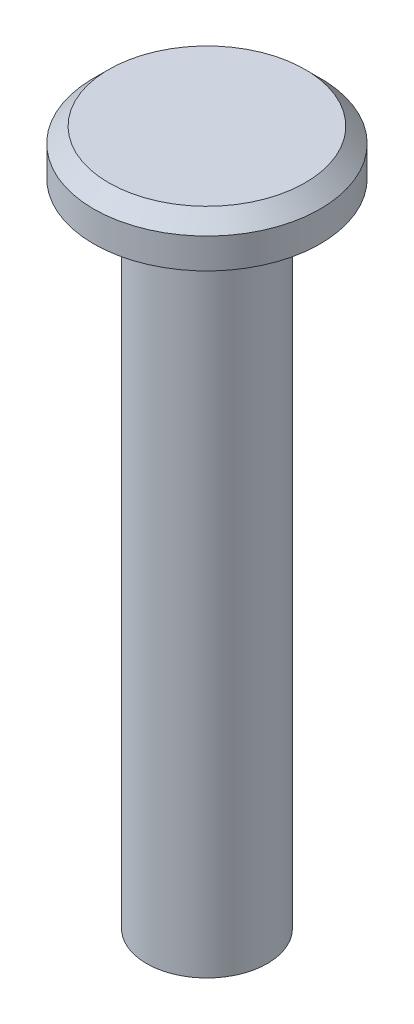
SolidWorks part; units mm, degrees
material "Plain Carbon Steel"
ref_plane "Front Plane" through (0, 0, 0) normal (0, 0, 1) x (1, 0, 0)
ref_plane "Top Plane" through (0, 0, 0) normal (0, 1, 0) x (1, 0, 0)
ref_plane "Right Plane" through (0, 0, 0) normal (1, 0, 0) x (0, 0, -1)
sketch "Shank Profile Ø8" plane through (0, 0, 0) normal (0, 1, 0) x (1, 0, 0)
  circle A0 centre (0, 0) radius 4
  dimension "D1" = 8
extrude "Shank Ø8x43" add sketch "Shank Profile Ø8" along normal blind 43
sketch "Head Profile Ø15" plane through (0, 43, 0) normal (0, 1, 0) x (1, 0, 0)
  circle A0 centre (0, 0) radius 7.5
  dimension "D1" = 15
extrude "Head Ø15x3" add sketch "Head Profile Ø15" along normal blind 3
chamfer "Head Edge Chamfer 1x45°" distance 1 angle 45 1 edges at (0, 46, 7.5)
